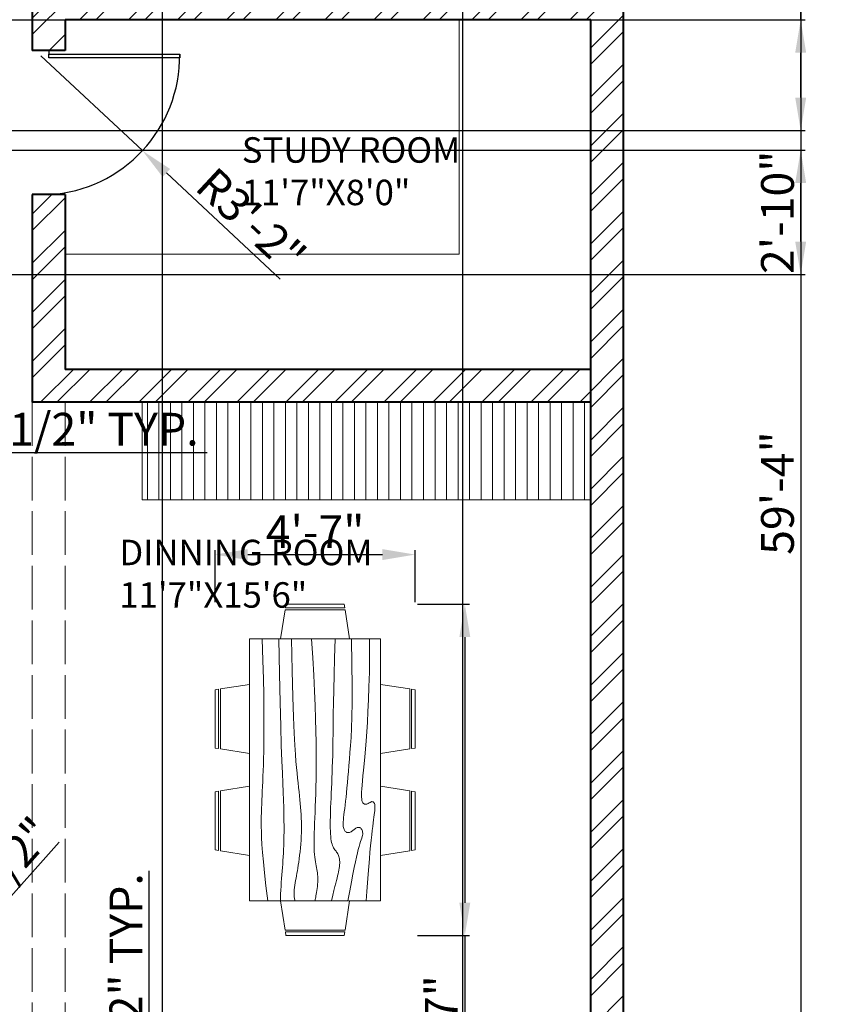
# Model space of a CAD drawing. Units: inches. Extents: x 3815 to 4442, y 1449 to 2534.
# Tile 4 of 5: x 4205 to 4428, y 1850 to 2120. Entities that reach past the tile are written whole.
import ezdxf

# ---------------------------------------------------------------- set-up
doc = ezdxf.new("R2010")
doc.units = ezdxf.units.IN
doc.linetypes.add('ACAD_ISO02W100', pattern=[15, 12, -3])
for name, color, linetype, lineweight in [('A-ANNO-DIMS', 2, 'Continuous', 18), ('A-AREA-IDEN', 7, 'Continuous', 20), ('A-DOOR', 4, 'Continuous', 25), ('A-FLOR-FIXD', 9, 'Continuous', 20), ('A-FLOR-PATT', 9, 'Continuous', 13), ('A-FURN', 8, 'Continuous', 18), ('A-WALL', 7, 'Continuous', 40), ('A-WALL-OVHD', 8, 'ACAD_ISO02W100', 18), ('A-WALL-PATT', 8, 'Continuous', 13), ('L-PLNT-PATT', 9, 'Continuous', 13)]:
    doc.layers.add(name, color=color, linetype=linetype, lineweight=lineweight)
doc.styles.get("Standard").update_dxf_attribs({"font": 'arial.ttf'})
doc.dimstyles.new('ISO-25', dxfattribs={"dimtxt": 9, "dimasz": 9, "dimexe": 1.25, "dimexo": 0.625, "dimtad": 1, "dimdec": 1, "dimrnd": 9, "dimlunit": 3, "dimtxsty": 'Standard', "dimcen": 2.5, "dimadec": 0, "dimazin": 0, "dimtfac": 1, "dimtdec": 1, "dimtmove": 0, "dimatfit": 3, "dimfxl": 1, "dimarcsym": 0})

# ---------------------------------------------------------------- blocks, each defined once
blk = doc.blocks.new('Dining Set - 36 x 72 in.')
for p, q in [((-22, 27.5), (-22.1562, 26.50042)), ((-22, 27.5), (-6, 27.5)), ((-5.8437, 26.49966), (-6, 27.5)), ((6, 27.5), (5.8438, 26.50042)), ((6, 27.5), (22, 27.5)), ((22.1563, 26.49966), (22, 27.5)), ((-22.2343, 26.00059), (-23.4847, 17.99762)), ((-22.2304, 26), (-5.7608, 26)), ((-5.8416, 26.5), (-22.1534, 26.5)), ((-4.5152, 17.99762), (-5.7655, 25.99926)), ((5.7657, 26.00059), (4.5153, 17.99762)), ((5.7696, 26), (22.2392, 26)), ((22.1584, 26.5), (5.8466, 26.5)), ((23.4848, 17.99762), (22.2345, 25.99926)), ((36, 18), (-36, 18)), ((-36, 18), (-36, -18)), ((36, -18), (36, 18)), ((-45.5, 8), (-44.5004, 8.15617)), ((-44.5, -8.15843), (-44.5, 8.15338)), ((-44.0006, 8.23428), (-35.9976, 9.48474)), ((-44, 8.23041), (-44, -8.23915)), ((44.0006, 8.23428), (35.9976, 9.48474)), ((44, 8.23041), (44, -8.23915)), ((44.5, -8.15843), (44.5, 8.15338)), ((45.5, 8), (44.5005, 8.15617)), ((-45.5, 8), (-45.5, -8)), ((45.5, 8), (45.5, -8)), ((-44.4997, -8.15631), (-45.5, -8)), ((44.4997, -8.15631), (45.5, -8)), ((-35.9976, -9.48476), (-43.9993, -8.2345)), ((35.9976, -9.48476), (43.9993, -8.2345)), ((-36, -18), (36, -18)), ((-22.2343, -26.0006), (-23.4847, -17.99762)), ((-4.5152, -17.99762), (-5.7655, -25.99928)), ((5.7657, -26.0006), (4.5153, -17.99762)), ((23.4848, -17.99762), (22.2345, -25.99928)), ((-22.2304, -26), (-5.7608, -26)), ((-22, -27.5), (-22.1562, -26.50044)), ((-5.8416, -26.5), (-22.1534, -26.5)), ((-5.8437, -26.49967), (-6, -27.5)), ((5.7696, -26), (22.2392, -26)), ((6, -27.5), (5.8438, -26.50044)), ((22.1584, -26.5), (5.8466, -26.5)), ((22.1563, -26.49967), (22, -27.5)), ((-22, -27.5), (-6, -27.5)), ((6, -27.5), (22, -27.5))]:
    blk.add_line(p, q)
for points in [[(-36, 15), (-31.1772, 14.97754), (-26.8079, 14.91406), (-22.8538, 14.81543), (-19.276, 14.6875), (-16.0362, 14.53613), (-13.0957, 14.36718), (-10.4159, 14.18652), (-7.9583, 14), (-5.6904, 13.81315), (-3.6035, 13.63021), (-1.6954, 13.45508), (0.0365, 13.29166), (1.5945, 13.14388), (2.9811, 13.01562), (4.1988, 12.9108), (5.25, 12.83333), (6.1393, 12.78613), (6.8802, 12.76823), (7.4883, 12.77767), (7.9792, 12.8125), (8.3685, 12.87077), (8.6719, 12.95052), (8.9049, 13.0498), (9.0833, 13.16666), (9.2205, 13.29899), (9.3216, 13.44401), (9.3895, 13.59879), (9.4271, 13.76041), (9.4373, 13.92594), (9.4232, 14.09245), (9.3875, 14.257), (9.3333, 14.41666), (9.2638, 14.56917), (9.1836, 14.71484), (9.0975, 14.85465), (9.0104, 14.98958), (8.9272, 15.1206), (8.8529, 15.2487), (8.7922, 15.37483), (8.75, 15.5), (8.7305, 15.62467), (8.7344, 15.74739), (8.7617, 15.86621), (8.8125, 15.97916), (8.8867, 16.08431), (8.9844, 16.17968), (9.1055, 16.26334), (9.25, 16.33333), (9.4189, 16.38802), (9.6172, 16.42708), (9.8506, 16.45052), (10.125, 16.45833), (10.4463, 16.45052), (10.8203, 16.42708), (11.2529, 16.38802), (11.75, 16.33333), (12.3184, 16.26318), (12.9694, 16.17838), (13.7151, 16.07991), (14.5677, 15.96875), (15.5395, 15.84586), (16.6426, 15.71224), (17.8893, 15.56884), (19.2917, 15.41666), (20.859, 15.25667), (22.5879, 15.08984), (24.4721, 14.91715), (26.5052, 14.73958), (28.6809, 14.5581), (30.9929, 14.3737), (33.4347, 14.18733), (36, 14)], [(-36, 10), (-28.9766, 10.14274), (-23.1725, 10.20442), (-18.4241, 10.19775), (-14.5677, 10.13541), (-11.4399, 10.03011), (-8.877, 9.89453), (-6.7154, 9.74137), (-4.7917, 9.58333), (-2.9698, 9.43082), (-1.2246, 9.28515), (0.4415, 9.14534), (2.026, 9.01041), (3.5266, 8.87939), (4.9408, 8.7513), (6.266, 8.62516), (7.5, 8.5), (8.6411, 8.37549), (9.6914, 8.2539), (10.6538, 8.13818), (11.5312, 8.03125), (12.3267, 7.93603), (13.043, 7.85547), (13.6831, 7.79248), (14.25, 7.75), (14.7471, 7.7303), (15.1797, 7.73307), (15.5537, 7.75732), (15.875, 7.80208), (16.1494, 7.86637), (16.3828, 7.94922), (16.5811, 8.04964), (16.75, 8.16666), (16.8944, 8.29915), (17.0143, 8.44531), (17.1089, 8.60319), (17.1771, 8.77083), (17.218, 8.94629), (17.2305, 9.1276), (17.2137, 9.31282), (17.1667, 9.5), (17.0895, 9.6875), (16.987, 9.875), (16.8649, 10.0625), (16.7292, 10.25), (16.5856, 10.4375), (16.4401, 10.625), (16.2985, 10.8125), (16.1667, 11), (16.05, 11.18733), (15.9518, 11.3737), (15.8752, 11.5581), (15.8229, 11.73958), (15.798, 11.91715), (15.8034, 12.08984), (15.842, 12.25667), (15.9167, 12.41666), (16.0295, 12.56836), (16.1784, 12.70833), (16.3605, 12.83268), (16.5729, 12.9375), (16.8127, 13.01888), (17.0768, 13.07291), (17.3625, 13.0957), (17.6667, 13.08333), (17.9894, 13.03312), (18.3418, 12.94726), (18.7382, 12.82918), (19.1927, 12.68229), (19.7195, 12.51001), (20.3327, 12.31575), (21.0465, 12.10294), (21.875, 11.875), (22.8357, 11.63354), (23.959, 11.37304), (25.2786, 11.08618), (26.8282, 10.76562), (28.6414, 10.40405), (30.752, 9.99414), (33.1936, 9.52856), (36, 9)], [(-36, 5.5), (-30.7157, 5.3348), (-26.069, 5.20963), (-21.9946, 5.11767), (-18.4271, 5.05208), (-15.3009, 5.00602), (-12.5508, 4.97265), (-10.1112, 4.94515), (-7.9167, 4.91666), (-5.909, 4.88167), (-4.0586, 4.83984), (-2.3429, 4.79215), (-0.7396, 4.73958), (0.7739, 4.6831), (2.22, 4.6237), (3.6213, 4.56233), (5, 4.5), (6.373, 4.43782), (7.7344, 4.3776), (9.0723, 4.32129), (10.375, 4.27083), (11.6309, 4.22819), (12.8281, 4.19531), (13.9551, 4.17415), (15, 4.16666), (15.954, 4.17448), (16.819, 4.19791), (17.6001, 4.23698), (18.3021, 4.29166), (18.9299, 4.36198), (19.4883, 4.44791), (19.9823, 4.54948), (20.4167, 4.66666), (20.7969, 4.79899), (21.1302, 4.94401), (21.4245, 5.09879), (21.6875, 5.26041), (21.9271, 5.42594), (22.1511, 5.59245), (22.3672, 5.757), (22.5834, 5.91666), (22.8065, 6.06868), (23.0404, 6.21093), (23.2879, 6.34147), (23.5521, 6.45833), (23.8358, 6.55957), (24.142, 6.64323), (24.4735, 6.70735), (24.8334, 6.75), (25.2235, 6.76969), (25.642, 6.76692), (26.0858, 6.74267), (26.5521, 6.69791), (27.0379, 6.63362), (27.5404, 6.55078), (28.0565, 6.45036), (28.5834, 6.33333), (29.1242, 6.19987), (29.7071, 6.04687), (30.3661, 5.87044), (31.1354, 5.66666), (32.0493, 5.43164), (33.142, 5.16146), (34.4475, 4.85221), (36, 4.5)], [(-36, -1), (-30.7915, -0.6591), (-26.0195, -0.38216), (-21.6519, -0.16284), (-17.6563, 0.00521), (-14.0005, 0.12833), (-10.6523, 0.21289), (-7.5796, 0.26522), (-4.75, 0.29166), (-2.134, 0.29793), (0.2878, 0.28711), (2.5317, 0.26163), (4.6146, 0.22396), (6.5529, 0.17651), (8.3633, 0.12174), (10.0623, 0.06209), (11.6667, 0), (13.1899, -0.06201), (14.6341, -0.1211), (15.9982, -0.17432), (17.2813, -0.21875), (18.4823, -0.25147), (19.6003, -0.26953), (20.6343, -0.27002), (21.5834, -0.25), (22.4481, -0.20768), (23.2357, -0.14584), (23.9549, -0.06836), (24.6146, 0.02083), (25.2235, 0.11784), (25.7904, 0.21875), (26.3241, 0.31966), (26.8334, 0.41666), (27.3265, 0.50618), (27.8099, 0.58593), (28.2894, 0.65397), (28.7709, 0.70833), (29.2601, 0.74707), (29.763, 0.76823), (30.2855, 0.76985), (30.8334, 0.75), (31.4088, 0.70784), (31.9994, 0.64713), (32.589, 0.57275), (33.1615, 0.48958), (33.7008, 0.4025), (34.1908, 0.3164), (34.6153, 0.23616), (34.9584, 0.16666), (35.2099, 0.11165), (35.3848, 0.07031), (35.504, 0.04069), (35.5886, 0.02083), (35.6594, 0.00879), (35.7377, 0.0026), (35.8442, 0.00032), (36, 0)], [(-36, -6.5), (-27.1843, -6.31267), (-20.084, -6.1263), (-14.469, -5.9419), (-10.1094, -5.76042), (-6.7752, -5.58285), (-4.2363, -5.41016), (-2.2629, -5.24333), (-0.625, -5.08334), (0.8708, -4.93099), (2.2715, -4.78646), (3.5872, -4.64974), (4.8281, -4.52084), (6.0046, -4.39974), (7.127, -4.28646), (8.2053, -4.18099), (9.25, -4.08334), (10.2705, -3.99382), (11.2734, -3.91407), (12.2647, -3.84603), (13.25, -3.79167), (14.2354, -3.75293), (15.2266, -3.73177), (16.2295, -3.73015), (17.25, -3.75), (18.2912, -3.79248), (19.3451, -3.85547), (20.4009, -3.93604), (21.4479, -4.03125), (22.4754, -4.13819), (23.4727, -4.25391), (24.4289, -4.37549), (25.3334, -4.5), (26.1785, -4.62492), (26.9694, -4.74935), (27.7145, -4.87281), (28.4219, -4.99479), (29.1, -5.11483), (29.7572, -5.23242), (30.4016, -5.34709), (31.0417, -5.45834), (31.6837, -5.56437), (32.3262, -5.65821), (32.9658, -5.73153), (33.599, -5.77604), (34.2224, -5.78345), (34.8327, -5.74545), (35.4264, -5.65373), (36, -5.5)], [(-36, -10), (-26.4022, -9.81299), (-18.4675, -9.62891), (-11.9839, -9.45069), (-6.7396, -9.28125), (-2.5226, -9.12354), (0.8789, -8.98047), (3.6769, -8.85498), (6.0833, -8.75), (8.2767, -8.66765), (10.3021, -8.60677), (12.1712, -8.56543), (13.8958, -8.54167), (15.4876, -8.53353), (16.9583, -8.53907), (18.3197, -8.55632), (19.5834, -8.58334), (20.7616, -8.61841), (21.8685, -8.66081), (22.9188, -8.71004), (23.9271, -8.76563), (24.9081, -8.82707), (25.8763, -8.89388), (26.8465, -8.96558), (27.8334, -9.04167), (28.8474, -9.12118), (29.8828, -9.20117), (30.93, -9.27824), (31.9792, -9.34896), (33.0205, -9.40991), (34.0443, -9.45768), (35.0407, -9.48885), (36, -9.5)], [(-36, -14.5), (-30.0881, -14.33513), (-25.0332, -14.21224), (-20.7312, -14.12647), (-17.0781, -14.07292), (-13.97, -14.04671), (-11.3027, -14.04297), (-8.9724, -14.05681), (-6.875, -14.08334), (-4.9224, -14.11833), (-3.0905, -14.16016), (-1.3709, -14.20785), (0.2448, -14.26042), (1.7647, -14.3169), (3.1973, -14.3763), (4.5507, -14.43767), (5.8333, -14.5), (7.0554, -14.5621), (8.235, -14.62175), (9.3922, -14.67652), (10.5469, -14.72396), (11.7192, -14.76164), (12.929, -14.78711), (14.1965, -14.79794), (15.5417, -14.79167), (16.9933, -14.76424), (18.6152, -14.70508), (20.4804, -14.60197), (22.6615, -14.44271), (25.2312, -14.21509), (28.2624, -13.9069), (31.8277, -13.50594), (36, -13)]]:
    blk.add_lwpolyline(points)
blk = doc.blocks.new('DOOR-LEAF-36IN')
for p, q in [((36, 2), (0, 2)), ((0, 2), (0, 1)), ((0, 0), (0, 1)), ((0, 1), (36, 1)), ((36, 1), (36, 2))]:
    blk.add_line(p, q)
blk = doc.blocks.new('*D21')
at = {"layer": 'A-ANNO-DIMS', "color": 0, "lineweight": -2, "transparency": 16777216}
for p, q in [((4240.73, 1821.3), (4240.73, 1886.41)), ((4237.75, 1812.3), (4241.98, 1812.3)), ((4237.75, 1810.3), (4241.98, 1810.3)), ((4240.73, 1810.3), (4240.73, 1812.3)), ((4240.73, 1801.3), (4240.73, 1792.3))]:
    blk.add_line(p, q, dxfattribs=at)
at = {"layer": 'A-ANNO-DIMS', "color": 0, "lineweight": 100, "transparency": 16777216}
for points in [[(4239.23, 1821.3), (4242.23, 1821.3), (4240.73, 1812.3)], [(4239.23, 1801.3), (4242.23, 1801.3), (4240.73, 1810.3)]]:
    blk.add_solid(points, dxfattribs=at)
at = {"layer": 'Defpoints', "color": 0, "lineweight": 100, "transparency": 16777216}
for p in [(4237.13, 1812.3), (4237.13, 1810.3), (4240.73, 1812.3)]:
    blk.add_point(p, dxfattribs=at)
at = {"layer": 'A-ANNO-DIMS', "color": 0, "transparency": 16777216, "insert": (4235.51, 1858.35), "char_height": 9, "attachment_point": 5, "rotation": 90}
blk.add_mtext('0\'-2" TYP.', dxfattribs=at)
blk = doc.blocks.new('*D40')
at = {"layer": 'A-ANNO-DIMS', "color": 0, "lineweight": -2, "transparency": 16777216}
for p, q in [((4106.2, 2000.57), (4106.2, 2002.6)), ((4115.53, 2000.57), (4115.53, 2002.6)), ((4097.2, 2001.35), (4088.2, 2001.35)), ((4106.2, 2001.35), (4115.53, 2001.35)), ((4124.53, 2001.35), (4256.68, 2001.35))]:
    blk.add_line(p, q, dxfattribs=at)
at = {"layer": 'A-ANNO-DIMS', "color": 0, "lineweight": 100, "transparency": 16777216}
for points in [[(4097.2, 2002.85), (4097.2, 1999.85), (4106.2, 2001.35)], [(4124.53, 2002.85), (4124.53, 1999.85), (4115.53, 2001.35)]]:
    blk.add_solid(points, dxfattribs=at)
at = {"layer": 'Defpoints', "color": 0, "lineweight": 100, "transparency": 16777216}
for p in [(4106.2, 1999.95), (4115.53, 2001.35), (4115.53, 1999.95)]:
    blk.add_point(p, dxfattribs=at)
at = {"layer": 'A-ANNO-DIMS', "color": 0, "transparency": 16777216, "insert": (4195.11, 2006.63), "char_height": 9, "attachment_point": 5}
blk.add_mtext('STOOL 0\'-9 1/2" TYP.', dxfattribs=at)
blk = doc.blocks.new('*D46')
at = {"layer": 'A-ANNO-DIMS', "color": 0, "lineweight": -2, "transparency": 16777216}
for p, q in [((4314.45, 1959.69), (4328.73, 1959.69)), ((4327.48, 1950.69), (4327.48, 1877.69)), ((4314.45, 1868.69), (4328.73, 1868.69)), ((4327.48, 1868.69), (4327.48, 1759.52))]:
    blk.add_line(p, q, dxfattribs=at)
at = {"layer": 'A-ANNO-DIMS', "color": 0, "lineweight": 100, "transparency": 16777216}
for points in [[(4325.98, 1950.69), (4328.98, 1950.69), (4327.48, 1959.69)], [(4325.98, 1877.69), (4328.98, 1877.69), (4327.48, 1868.69)]]:
    blk.add_solid(points, dxfattribs=at)
at = {"layer": 'Defpoints', "color": 0, "lineweight": 100, "transparency": 16777216}
for p in [(4313.83, 1959.69), (4313.83, 1868.69), (4327.48, 1868.69)]:
    blk.add_point(p, dxfattribs=at)
at = {"layer": 'A-ANNO-DIMS', "color": 0, "transparency": 16777216, "insert": (4322.2, 1809.6), "char_height": 9, "attachment_point": 5, "rotation": 90}
blk.add_mtext('DINING SET 7\'-7"', dxfattribs=at)
blk = doc.blocks.new('*D47')
at = {"layer": 'A-ANNO-DIMS', "color": 0, "lineweight": -2, "transparency": 16777216}
for p, q in [((4258.83, 1960.31), (4258.83, 1974.59)), ((4267.83, 1973.34), (4304.83, 1973.34)), ((4313.83, 1960.31), (4313.83, 1974.59))]:
    blk.add_line(p, q, dxfattribs=at)
at = {"layer": 'A-ANNO-DIMS', "color": 0, "lineweight": 100, "transparency": 16777216}
for points in [[(4267.83, 1974.84), (4267.83, 1971.84), (4258.83, 1973.34)], [(4304.83, 1974.84), (4304.83, 1971.84), (4313.83, 1973.34)]]:
    blk.add_solid(points, dxfattribs=at)
at = {"layer": 'Defpoints', "color": 0, "lineweight": 100, "transparency": 16777216}
for p in [(4313.83, 1973.34), (4258.83, 1959.69), (4313.83, 1959.69)]:
    blk.add_point(p, dxfattribs=at)
at = {"layer": 'A-ANNO-DIMS', "color": 0, "transparency": 16777216, "insert": (4286.33, 1978.46), "char_height": 9, "attachment_point": 5}
blk.add_mtext('4\'-7"', dxfattribs=at)
blk = doc.blocks.new('*D52')
at = {"layer": 'A-ANNO-DIMS', "color": 0, "lineweight": -2, "transparency": 16777216}
for p, q in [((4371.75, 2346.24), (4421.03, 2346.24)), ((4419.78, 2337.24), (4419.78, 1643.24)), ((4371.75, 1634.24), (4421.03, 1634.24))]:
    blk.add_line(p, q, dxfattribs=at)
at = {"layer": 'A-ANNO-DIMS', "color": 0, "lineweight": 100, "transparency": 16777216}
for points in [[(4418.28, 2337.24), (4421.28, 2337.24), (4419.78, 2346.24)], [(4418.28, 1643.24), (4421.28, 1643.24), (4419.78, 1634.24)]]:
    blk.add_solid(points, dxfattribs=at)
at = {"layer": 'Defpoints', "color": 0, "lineweight": 100, "transparency": 16777216}
for p in [(4371.13, 2346.24), (4371.13, 1634.24), (4419.78, 1634.24)]:
    blk.add_point(p, dxfattribs=at)
at = {"layer": 'A-ANNO-DIMS', "color": 0, "transparency": 16777216, "insert": (4414.56, 1990.24), "char_height": 9, "attachment_point": 5, "rotation": 90}
blk.add_mtext('59\'-4"', dxfattribs=at)
blk = doc.blocks.new('*D67')
at = {"layer": 'A-ANNO-DIMS', "color": 0, "lineweight": -2, "transparency": 16777216}
for p, q in [((4419.78, 2120.24), (4419.78, 2175.54)), ((3960.75, 2120.24), (4421.03, 2120.24)), ((4419.78, 2098.9), (4419.78, 2111.24)), ((3960.75, 2089.9), (4421.03, 2089.9))]:
    blk.add_line(p, q, dxfattribs=at)
at = {"layer": 'A-ANNO-DIMS', "color": 0, "lineweight": 100, "transparency": 16777216}
for points in [[(4418.28, 2111.24), (4421.28, 2111.24), (4419.78, 2120.24)], [(4418.28, 2098.9), (4421.28, 2098.9), (4419.78, 2089.9)]]:
    blk.add_solid(points, dxfattribs=at)
at = {"layer": 'Defpoints', "color": 0, "lineweight": 100, "transparency": 16777216}
for p in [(3960.13, 2120.24), (4419.78, 2120.24), (3960.13, 2089.9)]:
    blk.add_point(p, dxfattribs=at)
at = {"layer": 'A-ANNO-DIMS', "color": 0, "transparency": 16777216, "insert": (4414.5, 2152.39), "char_height": 9, "attachment_point": 5, "rotation": 90}
blk.add_mtext('2\'-6 1/2"', dxfattribs=at)
blk = doc.blocks.new('*D68')
at = {"layer": 'A-ANNO-DIMS', "color": 0, "lineweight": -2, "transparency": 16777216}
for p, q in [((4025.25, 2084.42), (4421.03, 2084.42)), ((4419.78, 2059.34), (4419.78, 2075.42)), ((4025.25, 2050.34), (4421.03, 2050.34))]:
    blk.add_line(p, q, dxfattribs=at)
at = {"layer": 'A-ANNO-DIMS', "color": 0, "lineweight": 100, "transparency": 16777216}
for points in [[(4418.28, 2075.42), (4421.28, 2075.42), (4419.78, 2084.42)], [(4418.28, 2059.34), (4421.28, 2059.34), (4419.78, 2050.34)]]:
    blk.add_solid(points, dxfattribs=at)
at = {"layer": 'Defpoints', "color": 0, "lineweight": 100, "transparency": 16777216}
for p in [(4024.63, 2084.42), (4419.78, 2084.42), (4024.63, 2050.34)]:
    blk.add_point(p, dxfattribs=at)
at = {"layer": 'A-ANNO-DIMS', "color": 0, "transparency": 16777216, "insert": (4414.56, 2067.38), "char_height": 9, "attachment_point": 5, "rotation": 90}
blk.add_mtext('2\'-10"', dxfattribs=at)
blk = doc.blocks.new('*D76')
at = {"layer": 'A-ANNO-DIMS', "color": 0, "lineweight": -2, "transparency": 16777216}
for p, q in [((4244.38, 1827.87), (4244.38, 2516.14)), ((4326.89, 1827.87), (4326.89, 2516.14)), ((4253.38, 2514.89), (4317.89, 2514.89))]:
    blk.add_line(p, q, dxfattribs=at)
at = {"layer": 'A-ANNO-DIMS', "color": 0, "lineweight": 100, "transparency": 16777216}
for points in [[(4253.38, 2516.39), (4253.38, 2513.39), (4244.38, 2514.89)], [(4317.89, 2516.39), (4317.89, 2513.39), (4326.89, 2514.89)]]:
    blk.add_solid(points, dxfattribs=at)
at = {"layer": 'Defpoints', "color": 0, "lineweight": 100, "transparency": 16777216}
for p in [(4326.89, 2514.89), (4244.38, 1827.24), (4326.89, 1827.24)]:
    blk.add_point(p, dxfattribs=at)
at = {"layer": 'A-ANNO-DIMS', "color": 0, "transparency": 16777216, "insert": (4285.63, 2520.17), "char_height": 9, "attachment_point": 5}
blk.add_mtext('6\'-10 1/2"', dxfattribs=at)
blk = doc.blocks.new('*D80')
at = {"layer": 'A-ANNO-DIMS', "color": 0, "lineweight": -2, "transparency": 16777216}
for p, q in [((4210.93, 2110.37), (4238.88, 2084.33)), ((4276.77, 2049.03), (4245.46, 2078.2))]:
    blk.add_line(p, q, dxfattribs=at)
at = {"layer": 'A-ANNO-DIMS', "color": 0, "lineweight": 100, "transparency": 16777216}
blk.add_solid([(4246.48, 2079.3), (4244.44, 2077.1), (4238.88, 2084.33)], dxfattribs=at)
at = {"layer": 'Defpoints', "color": 0, "lineweight": 100, "transparency": 16777216}
for p in [(4210.93, 2110.37), (4238.88, 2084.33)]:
    blk.add_point(p, dxfattribs=at)
at = {"layer": 'A-ANNO-DIMS', "color": 0, "transparency": 16777216, "insert": (4267.97, 2064.37), "char_height": 9, "attachment_point": 5, "rotation": 317.0203}
blk.add_mtext('R3\'-2"', dxfattribs=at)
blk = doc.blocks.new('*D90')
at = {"layer": 'A-ANNO-DIMS', "color": 0, "lineweight": -2, "transparency": 16777216}
for p, q in [((4215.97, 1894.31), (4173.53, 1846.73)), ((4149.88, 1820.22), (4167.53, 1840.01))]:
    blk.add_line(p, q, dxfattribs=at)
at = {"layer": 'A-ANNO-DIMS', "color": 0, "lineweight": 100, "transparency": 16777216}
blk.add_solid([(4172.41, 1847.73), (4174.65, 1845.73), (4167.53, 1840.01)], dxfattribs=at)
at = {"layer": 'Defpoints', "color": 0, "lineweight": 100, "transparency": 16777216}
for p in [(4167.53, 1840.01), (4149.88, 1820.22)]:
    blk.add_point(p, dxfattribs=at)
at = {"layer": 'A-ANNO-DIMS', "color": 0, "transparency": 16777216, "insert": (4193.8, 1877.39), "char_height": 9, "attachment_point": 5, "rotation": 48.2637}
blk.add_mtext('R2\'-2 1/2"', dxfattribs=at)

msp = doc.modelspace()

# ---------------------------------------------------------------- hatches: boundary and pattern name
at = {"layer": 'A-FLOR-PATT'}
h = msp.add_hatch(dxfattribs=at)
h.set_pattern_fill('ANSI31', color=256, scale=0.995904, angle=45, style=0)
h.paths.add_polyline_path([(4238.81, 1988.39), (4362.13, 1988.39), (4362.13, 2015.24), (4238.81, 2015.24)])
at = {"layer": 'A-WALL-PATT'}
h = msp.add_hatch(dxfattribs=at)
h.set_pattern_fill('ANSI32', color=256)
h.paths.add_polyline_path([(4156.29, 2346.24), (3989.15, 2346.24), (3989.15, 2337.24), (4044.13, 2337.24), (4044.13, 2305.59, -0.025534), (4046.38, 2305.51), (4048.63, 2305.51), (4048.63, 2337.24), (4139.63, 2337.24), (4139.63, 2277.24), (4112.45, 2277.24), (4112.45, 2272.74), (4139.63, 2272.74), (4139.63, 2180.66), (4148.63, 2180.66), (4148.63, 2184.24), (4208.63, 2184.24), (4208.63, 2180.66), (4213.13, 2180.66), (4213.13, 2209.79), (4208.63, 2209.79), (4208.63, 2188.74), (4148.63, 2188.74), (4148.63, 2254.74), (4185.97, 2254.74), (4185.97, 2259.24), (4148.63, 2259.24), (4148.63, 2337.24), (4156.29, 2337.24)])
h.paths.add_polyline_path([(4251.85, 2346.24), (4180.29, 2346.24), (4180.29, 2337.24), (4208.63, 2337.24), (4208.63, 2259.24), (4205.62, 2259.24), (4205.62, 2254.74), (4208.63, 2254.74), (4208.63, 2245.05), (4213.13, 2245.05), (4213.13, 2337.24), (4251.85, 2337.24)])
h.paths.add_polyline_path([(4371.13, 2346.24), (4311.85, 2346.24), (4311.85, 2337.24), (4362.13, 2337.24), (4362.13, 2129.24), (4213.13, 2129.24), (4213.13, 2137.97), (4208.63, 2137.97), (4208.63, 2111.87), (4217.63, 2111.87), (4217.63, 2120.24), (4362.13, 2120.24), (4362.13, 1643.24), (4318.71, 1643.24), (4318.71, 1634.24), (4371.13, 1634.24)])
h.paths.add_polyline_path([(3960.13, 2175.52), (3951.13, 2175.52), (3951.13, 2089.9), (3960.13, 2089.9), (3960.13, 2120.24), (4020.13, 2120.24), (4020.13, 2084.42), (4024.63, 2084.42), (4024.63, 2120.24), (4139.63, 2120.24), (4139.63, 2062.37), (4148.63, 2062.37), (4148.63, 2137.97), (4139.63, 2137.97), (4139.63, 2129.24), (3960.13, 2129.24)])
h.paths.add_polyline_path([(3960.13, 2272.74), (4044.13, 2272.74), (4079.8, 2272.74), (4079.8, 2277.24), (4048.63, 2277.24), (4048.63, 2282.04), (4044.13, 2282.04), (4044.13, 2277.24), (3960.13, 2277.24), (3960.13, 2337.24), (3965.15, 2337.24), (3965.15, 2346.24), (3951.13, 2346.24), (3951.13, 2235.52), (3960.13, 2235.52)])
h.paths.add_polyline_path([(4024.63, 2050.34), (4020.13, 2050.34), (4020.13, 2012.24), (3960.13, 2012.24), (3960.13, 2051.05), (3951.13, 2051.05), (3951.13, 1979.78), (3960.13, 1979.78), (3960.13, 2003.24), (4024.63, 2003.24)])
h.paths.add_polyline_path([(4217.63, 2072.24), (4208.63, 2072.24), (4208.63, 2015.24), (4362.13, 2015.24), (4362.13, 2024.24), (4217.63, 2024.24)], flags=17)
h.paths.add_polyline_path([(3960.13, 1940.92), (3951.13, 1940.92), (3951.13, 1883.13), (3960.13, 1883.13)])
h.paths.add_polyline_path([(3960.13, 1822.74), (4149.38, 1822.74), (4149.38, 1827.24), (3960.13, 1827.24), (3960.13, 1844.28), (3951.13, 1844.28), (3951.13, 1769.4), (3960.13, 1769.4)])
h.paths.add_polyline_path([(4362.13, 1827.24), (4326.89, 1827.24), (4326.89, 1818.24), (4362.13, 1818.24)], flags=17)
h.paths.add_polyline_path([(4244.38, 1827.24), (4208.63, 1827.24), (4203.18, 1827.24), (4203.18, 1822.74), (4208.63, 1822.74), (4208.63, 1812.3), (4217.63, 1812.3), (4217.63, 1818.24), (4244.38, 1818.24)])
h.paths.add_polyline_path([(4149.38, 1738.74), (4142.66, 1738.74), (4142.66, 1742.16), (4138.16, 1742.16), (4138.16, 1738.74), (4090.16, 1738.74), (4090.16, 1774.74), (4138.16, 1774.74), (4138.16, 1763.78), (4142.66, 1763.78), (4142.66, 1774.74), (4142.66, 1779.24), (4138.16, 1779.24), (4090.16, 1779.24), (4085.66, 1779.24), (4085.66, 1774.74), (4085.66, 1738.74), (3960.13, 1738.74), (3960.13, 1743.46), (3951.13, 1743.46), (3951.13, 1729.74), (4149.38, 1729.74)])
h.paths.add_polyline_path([(4136.7, 1703.49), (4136.7, 1729.74), (4127.7, 1729.74), (4127.7, 1703.49), (4127.7, 1701.02), (4181.38, 1655.79), (4183.63, 1655.79), (4208.63, 1655.79), (4208.63, 1664.79), (4183.63, 1664.79)])
h.paths.add_polyline_path([(4217.63, 1771.49), (4208.63, 1771.49), (4208.63, 1738.74), (4202.94, 1738.74), (4202.94, 1729.74), (4208.63, 1729.74), (4208.63, 1634.24), (4258.71, 1634.24), (4258.71, 1643.24), (4217.63, 1643.24)])
at = {"layer": 'L-PLNT-PATT'}
h = msp.add_hatch(dxfattribs=at)
h.set_pattern_fill('GOST_GLASS', color=256)
h.paths.add_polyline_path([(4368.13, 2463.24), (3894.13, 2463.24, -0.246049), (3960.13, 2346.24), (4368.13, 2346.24)])
h.paths.add_polyline_path([(4365.15, 1631.83), (4112.05, 1631.83), (4112.05, 1581.3), (4365.15, 1581.3)])
h.paths.add_polyline_path([(4365.15, 1581.3), (4112.05, 1581.3), (4112.05, 1511.54), (4365.15, 1511.54)])
h.paths.add_polyline_path([(4219.4, 1545.72), (4287.81, 1545.72), (4287.81, 1571.84), (4219.4, 1571.84)], flags=24)

# ---------------------------------------------------------------- linework, layer by layer
at = {"layer": 'A-DOOR'}
msp.add_arc((4210.93, 2110.37), 38.2, 273.2914, 0.75, dxfattribs=at)
at = {"layer": 'A-FLOR-FIXD'}
for p, q in [((4325.96, 2055.87), (4325.96, 2120.24)), ((4217.63, 2055.87), (4325.96, 2055.87)), ((4238.81, 1988.39), (4238.81, 2015.24)), ((4362.13, 1988.39), (4238.81, 1988.39))]:
    msp.add_line(p, q, dxfattribs=at)
at = {"layer": 'A-WALL'}
for p, q in [((4371.13, 1634.24), (4371.13, 2346.24)), ((4208.63, 2137.97), (4208.63, 2111.87)), ((4362.13, 2120.24), (4217.63, 2120.24)), ((4217.63, 2120.24), (4217.63, 2111.87)), ((4362.13, 1643.24), (4362.13, 2120.24)), ((4217.63, 2111.87), (4208.63, 2111.87)), ((4217.63, 2072.24), (4208.63, 2072.24)), ((4208.63, 2072.24), (4208.63, 2015.24)), ((4217.63, 2072.24), (4217.63, 2024.24)), ((4362.13, 2024.24), (4217.63, 2024.24)), ((4362.13, 2015.24), (4208.63, 2015.24))]:
    msp.add_line(p, q, dxfattribs=at)
at = {"layer": 'A-WALL-OVHD'}
for p, q in [((4208.63, 2015.24), (4208.63, 1827.24)), ((4217.63, 2015.24), (4217.63, 1827.24))]:
    msp.add_line(p, q, dxfattribs=at)

# ---------------------------------------------------------------- block references
at = {"layer": 'A-DOOR', "extrusion": (0, 0, -1), "zscale": -1, "rotation": 180}
msp.add_blockref('DOOR-LEAF-36IN', (-4213.13, 2111.87), dxfattribs=at)
at = {"layer": 'A-FURN', "rotation": 270}
msp.add_blockref('Dining Set - 36 x 72 in.', (4286.33, 1914.19), dxfattribs=at)

# ---------------------------------------------------------------- texts
at = {"layer": 'A-AREA-IDEN', "char_height": 7, "attachment_point": 1}
for s, width, insert in [('STUDY ROOM\\P11\'7"X8\'0"', 81.473, (4266.18, 2088.01)), ('DINNING ROOM\\P11\'7"X15\'6"', 100.9984, (4232.54, 1977.42))]:
    msp.add_mtext_dynamic_manual_height_columns(s, width=width, gutter_width=12.5, heights=[0], dxfattribs=dict(at, insert=insert))

# ---------------------------------------------------------------- dimensions: what is measured, and where the dimension line sits
at = {"layer": 'A-ANNO-DIMS'}
for base, p1, p2, picture, middle in [((4326.89, 2514.89), (4244.38, 1827.24), (4326.89, 1827.24), '*D76', (4285.63, 2520.17)), ((4313.83, 1973.34), (4258.83, 1959.69), (4313.83, 1959.69), '*D47', (4286.33, 1978.46))]:
    dim = msp.add_linear_dim(base=base, p1=p1, p2=p2, dimstyle='ISO-25', override={"dimdec": 1, "dimlfac": 1, "dimrnd": 0, "dimzin": 1, "dimdsep": 46, "dimlunit": 4, "dimfrac": 2}, dxfattribs=at)
    dim.commit()
    dim.dimension.update_dxf_attribs({"geometry": picture, "text_midpoint": middle})
for base, p1, p2, picture, middle in [((4419.78, 1634.24), (4371.13, 2346.24), (4371.13, 1634.24), '*D52', (4414.56, 1990.24)), ((4419.78, 2120.24), (3960.13, 2089.9), (3960.13, 2120.24), '*D67', (4414.5, 2152.39)), ((4419.78, 2084.42), (4024.63, 2050.34), (4024.63, 2084.42), '*D68', (4414.56, 2067.38))]:
    dim = msp.add_linear_dim(base=base, p1=p1, p2=p2, angle=90, dimstyle='ISO-25', override={"dimdec": 1, "dimlfac": 1, "dimrnd": 0, "dimzin": 1, "dimdsep": 46, "dimlunit": 4, "dimfrac": 2}, dxfattribs=at)
    dim.commit()
    dim.dimension.update_dxf_attribs({"geometry": picture, "text_midpoint": middle})
for center, mpoint, picture, middle in [((4210.93, 2110.37), (4238.88, 2084.33), '*D80', (4267.97, 2064.37)), ((4149.88, 1820.22), (4167.53, 1840.01), '*D90', (4193.8, 1877.39))]:
    dim = msp.add_radius_dim(center=center, mpoint=mpoint, dimstyle='ISO-25', override={"dimdec": 1, "dimlfac": 1, "dimrnd": 0, "dimzin": 1, "dimdsep": 46, "dimlunit": 4, "dimfrac": 2}, dxfattribs=at)
    dim.commit()
    dim.dimension.update_dxf_attribs({"geometry": picture, "text_midpoint": middle})
dim = msp.add_linear_dim(base=(4115.53, 2001.35), p1=(4106.2, 1999.95), p2=(4115.53, 1999.95), text='STOOL <> TYP.', dimstyle='ISO-25', override={"dimdec": 1, "dimlfac": 1, "dimrnd": 0, "dimzin": 1, "dimdsep": 46, "dimlunit": 4, "dimfrac": 2}, dxfattribs=at)
dim.commit()
dim.dimension.update_dxf_attribs({"geometry": '*D40', "text_midpoint": (4195.11, 2006.63)})
for base, p1, p2, angle, text, picture, middle in [((4327.48, 1868.69), (4313.83, 1959.69), (4313.83, 1868.69), 270, 'DINING SET <>', '*D46', (4322.2, 1809.6)), ((4240.73, 1812.3), (4237.13, 1810.3), (4237.13, 1812.3), 90, '<> TYP.', '*D21', (4235.51, 1858.35))]:
    dim = msp.add_linear_dim(base=base, p1=p1, p2=p2, angle=angle, text=text, dimstyle='ISO-25', override={"dimdec": 1, "dimlfac": 1, "dimrnd": 0, "dimzin": 1, "dimdsep": 46, "dimlunit": 4, "dimfrac": 2}, dxfattribs=at)
    dim.commit()
    dim.dimension.update_dxf_attribs({"geometry": picture, "text_midpoint": middle})

doc.saveas('drawing.dxf')
